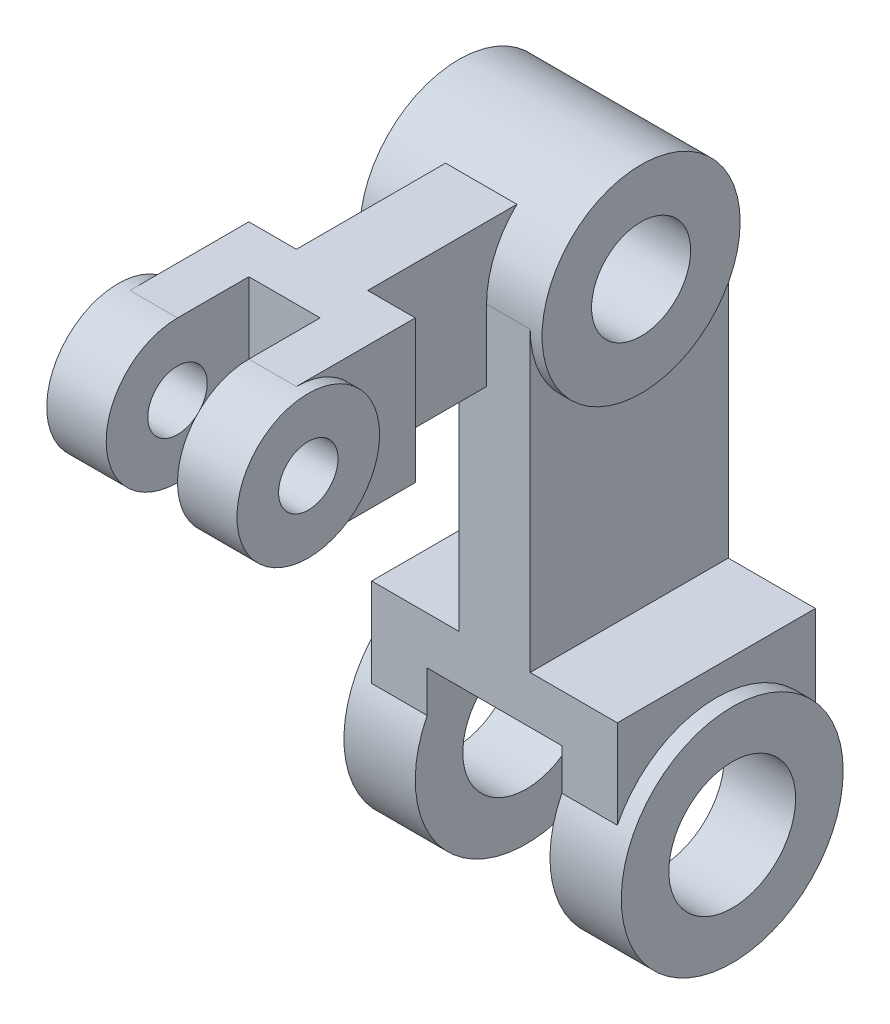
ISO-10303-21;
HEADER;
FILE_DESCRIPTION(('STEP AP214'),'2;1');
FILE_NAME('part.step','',(''),(''),'','','');
FILE_SCHEMA(('AUTOMOTIVE_DESIGN { 1 0 10303 214 1 1 1 1 }'));
ENDSEC;
DATA;
#1=APPLICATION_CONTEXT('core data for automotive mechanical design processes');
#2=APPLICATION_PROTOCOL_DEFINITION('international standard','automotive_design',2000,#1);
#3=PRODUCT_CONTEXT('',#1,'mechanical');
#4=PRODUCT('Part','Part','',(#3));
#5=PRODUCT_RELATED_PRODUCT_CATEGORY('part','',(#4));
#6=PRODUCT_DEFINITION_FORMATION('','',#4);
#7=PRODUCT_DEFINITION_CONTEXT('part definition',#1,'design');
#8=PRODUCT_DEFINITION('design','',#6,#7);
#9=PRODUCT_DEFINITION_SHAPE('','',#8);
#10=(LENGTH_UNIT() NAMED_UNIT(*) SI_UNIT(.MILLI.,.METRE.));
#11=(NAMED_UNIT(*) PLANE_ANGLE_UNIT() SI_UNIT($,.RADIAN.));
#12=(NAMED_UNIT(*) SI_UNIT($,.STERADIAN.) SOLID_ANGLE_UNIT());
#13=UNCERTAINTY_MEASURE_WITH_UNIT(LENGTH_MEASURE(1.E-05),#10,'distance_accuracy_value','');
#14=(GEOMETRIC_REPRESENTATION_CONTEXT(3) GLOBAL_UNCERTAINTY_ASSIGNED_CONTEXT((#13)) GLOBAL_UNIT_ASSIGNED_CONTEXT((#10,
#11,#12)) REPRESENTATION_CONTEXT('',''));
#15=CARTESIAN_POINT('',(0.,0.,0.));
#16=DIRECTION('',(0.,0.,1.));
#17=DIRECTION('',(1.,0.,0.));
#18=AXIS2_PLACEMENT_3D('',#15,#16,#17);
#19=CARTESIAN_POINT('',(13.,110.,85.));
#20=DIRECTION('',(-1.,0.,0.));
#21=DIRECTION('',(0.,0.,1.));
#22=AXIS2_PLACEMENT_3D('',#19,#20,#21);
#23=CYLINDRICAL_SURFACE('',#22,18.);
#24=CARTESIAN_POINT('',(-35.,110.,85.));
#25=DIRECTION('',(1.,0.,0.));
#26=DIRECTION('',(0.,0.,-1.));
#27=AXIS2_PLACEMENT_3D('',#24,#25,#26);
#28=CIRCLE('',#27,18.);
#29=CARTESIAN_POINT('',(-35.,110.,67.));
#30=VERTEX_POINT('',#29);
#31=EDGE_CURVE('E451',#30,#30,#28,.T.);
#32=ORIENTED_EDGE('',*,*,#31,.T.);
#33=EDGE_LOOP('',(#32));
#34=FACE_BOUND('',#33,.T.);
#35=CARTESIAN_POINT('',(-32.,110.,85.));
#36=DIRECTION('',(-1.,0.,0.));
#37=DIRECTION('',(0.,0.,1.));
#38=AXIS2_PLACEMENT_3D('',#35,#36,#37);
#39=CIRCLE('',#38,18.);
#40=CARTESIAN_POINT('',(-32.,128.,85.));
#41=VERTEX_POINT('',#40);
#42=CARTESIAN_POINT('',(-32.,92.,85.));
#43=VERTEX_POINT('',#42);
#44=EDGE_CURVE('E448',#41,#43,#39,.T.);
#45=ORIENTED_EDGE('',*,*,#44,.T.);
#46=DIRECTION('',(1.,0.,0.));
#47=VECTOR('',#46,1.);
#48=CARTESIAN_POINT('',(-20.,92.,85.));
#49=LINE('',#48,#47);
#50=CARTESIAN_POINT('',(-20.,92.,85.));
#51=VERTEX_POINT('',#50);
#52=EDGE_CURVE('E382',#43,#51,#49,.T.);
#53=ORIENTED_EDGE('',*,*,#52,.T.);
#54=CARTESIAN_POINT('',(-20.,110.,85.));
#55=DIRECTION('',(-1.,0.,0.));
#56=DIRECTION('',(0.,0.,1.));
#57=AXIS2_PLACEMENT_3D('',#54,#55,#56);
#58=CIRCLE('',#57,18.);
#59=CARTESIAN_POINT('',(-20.,128.,85.));
#60=VERTEX_POINT('',#59);
#61=EDGE_CURVE('E51',#51,#60,#58,.T.);
#62=ORIENTED_EDGE('',*,*,#61,.T.);
#63=DIRECTION('',(1.,0.,0.));
#64=VECTOR('',#63,1.);
#65=CARTESIAN_POINT('',(-20.,128.,85.));
#66=LINE('',#65,#64);
#67=EDGE_CURVE('E410',#41,#60,#66,.T.);
#68=ORIENTED_EDGE('',*,*,#67,.F.);
#69=EDGE_LOOP('',(#45,#53,#62,#68));
#70=FACE_BOUND('',#69,.T.);
#71=ADVANCED_FACE('F50',(#34,#70),#23,.T.);
#72=CARTESIAN_POINT('',(13.,110.,85.));
#73=DIRECTION('',(-1.,0.,0.));
#74=DIRECTION('',(0.,0.,1.));
#75=AXIS2_PLACEMENT_3D('',#72,#73,#74);
#76=CYLINDRICAL_SURFACE('',#75,7.5);
#77=CARTESIAN_POINT('',(-20.,110.,85.));
#78=DIRECTION('',(-1.,0.,0.));
#79=DIRECTION('',(0.,0.,1.));
#80=AXIS2_PLACEMENT_3D('',#77,#78,#79);
#81=CIRCLE('',#80,7.5);
#82=CARTESIAN_POINT('',(-20.,110.,92.5));
#83=VERTEX_POINT('',#82);
#84=EDGE_CURVE('E11',#83,#83,#81,.T.);
#85=ORIENTED_EDGE('',*,*,#84,.F.);
#86=EDGE_LOOP('',(#85));
#87=FACE_BOUND('',#86,.T.);
#88=CARTESIAN_POINT('',(-35.,110.,85.));
#89=DIRECTION('',(1.,0.,0.));
#90=DIRECTION('',(0.,0.,-1.));
#91=AXIS2_PLACEMENT_3D('',#88,#89,#90);
#92=CIRCLE('',#91,7.5);
#93=CARTESIAN_POINT('',(-35.,110.,77.5));
#94=VERTEX_POINT('',#93);
#95=EDGE_CURVE('E57',#94,#94,#92,.T.);
#96=ORIENTED_EDGE('',*,*,#95,.F.);
#97=EDGE_LOOP('',(#96));
#98=FACE_BOUND('',#97,.T.);
#99=ADVANCED_FACE('F47',(#87,#98),#76,.F.);
#100=CARTESIAN_POINT('',(-35.,110.,85.));
#101=DIRECTION('',(1.,0.,0.));
#102=DIRECTION('',(0.,0.,-1.));
#103=AXIS2_PLACEMENT_3D('',#100,#101,#102);
#104=PLANE('',#103);
#105=ORIENTED_EDGE('',*,*,#31,.F.);
#106=EDGE_LOOP('',(#105));
#107=FACE_BOUND('',#106,.T.);
#108=ORIENTED_EDGE('',*,*,#95,.T.);
#109=EDGE_LOOP('',(#108));
#110=FACE_BOUND('',#109,.T.);
#111=ADVANCED_FACE('F488',(#107,#110),#104,.F.);
#112=CARTESIAN_POINT('',(-20.,-28.,67.));
#113=DIRECTION('',(-1.,0.,0.));
#114=DIRECTION('',(0.,0.,1.));
#115=AXIS2_PLACEMENT_3D('',#112,#113,#114);
#116=PLANE('',#115);
#117=ORIENTED_EDGE('',*,*,#84,.T.);
#118=EDGE_LOOP('',(#117));
#119=FACE_BOUND('',#118,.T.);
#120=ORIENTED_EDGE('',*,*,#61,.F.);
#121=DIRECTION('',(0.,0.,-1.));
#122=VECTOR('',#121,1.);
#123=CARTESIAN_POINT('',(-20.,92.,85.));
#124=LINE('',#123,#122);
#125=CARTESIAN_POINT('',(-20.,92.,67.));
#126=VERTEX_POINT('',#125);
#127=EDGE_CURVE('E381',#51,#126,#124,.T.);
#128=ORIENTED_EDGE('',*,*,#127,.T.);
#129=DIRECTION('',(0.,1.,0.));
#130=VECTOR('',#129,1.);
#131=CARTESIAN_POINT('',(-20.,92.,67.));
#132=LINE('',#131,#130);
#133=CARTESIAN_POINT('',(-20.,128.,67.));
#134=VERTEX_POINT('',#133);
#135=EDGE_CURVE('E436',#126,#134,#132,.T.);
#136=ORIENTED_EDGE('',*,*,#135,.T.);
#137=DIRECTION('',(0.,0.,-1.));
#138=VECTOR('',#137,1.);
#139=CARTESIAN_POINT('',(-20.,128.,85.));
#140=LINE('',#139,#138);
#141=EDGE_CURVE('E407',#60,#134,#140,.T.);
#142=ORIENTED_EDGE('',*,*,#141,.F.);
#143=EDGE_LOOP('',(#120,#128,#136,#142));
#144=FACE_BOUND('',#143,.T.);
#145=ADVANCED_FACE('F465',(#119,#144),#116,.F.);
#146=CARTESIAN_POINT('',(-20.,92.,14.9257157700794));
#147=DIRECTION('',(-1.,0.,0.));
#148=DIRECTION('',(0.,0.,1.));
#149=AXIS2_PLACEMENT_3D('',#146,#147,#148);
#150=PLANE('',#149);
#151=CARTESIAN_POINT('',(-20.,110.,0.));
#152=DIRECTION('',(-1.,0.,0.));
#153=DIRECTION('',(0.,0.,1.));
#154=AXIS2_PLACEMENT_3D('',#151,#152,#153);
#155=CIRCLE('',#154,25.);
#156=CARTESIAN_POINT('',(-20.,92.,17.3493515728975));
#157=VERTEX_POINT('',#156);
#158=CARTESIAN_POINT('',(-20.,128.,17.3493515728975));
#159=VERTEX_POINT('',#158);
#160=EDGE_CURVE('E354',#157,#159,#155,.T.);
#161=ORIENTED_EDGE('',*,*,#160,.F.);
#162=DIRECTION('',(0.,0.,1.));
#163=VECTOR('',#162,1.);
#164=CARTESIAN_POINT('',(-20.,92.,14.9257157700794));
#165=LINE('',#164,#163);
#166=CARTESIAN_POINT('',(-20.,92.,55.));
#167=VERTEX_POINT('',#166);
#168=EDGE_CURVE('E375',#157,#167,#165,.T.);
#169=ORIENTED_EDGE('',*,*,#168,.T.);
#170=DIRECTION('',(0.,1.,0.));
#171=VECTOR('',#170,1.);
#172=CARTESIAN_POINT('',(-20.,92.,55.));
#173=LINE('',#172,#171);
#174=CARTESIAN_POINT('',(-20.,128.,55.));
#175=VERTEX_POINT('',#174);
#176=EDGE_CURVE('E401',#167,#175,#173,.T.);
#177=ORIENTED_EDGE('',*,*,#176,.T.);
#178=DIRECTION('',(0.,0.,1.));
#179=VECTOR('',#178,1.);
#180=CARTESIAN_POINT('',(-20.,128.,14.9257157700794));
#181=LINE('',#180,#179);
#182=EDGE_CURVE('E371',#159,#175,#181,.T.);
#183=ORIENTED_EDGE('',*,*,#182,.F.);
#184=EDGE_LOOP('',(#161,#169,#177,#183));
#185=FACE_BOUND('',#184,.T.);
#186=ADVANCED_FACE('F493',(#185),#150,.T.);
#187=CARTESIAN_POINT('',(-2.,92.,14.9257157700794));
#188=DIRECTION('',(1.,0.,0.));
#189=DIRECTION('',(0.,0.,-1.));
#190=AXIS2_PLACEMENT_3D('',#187,#188,#189);
#191=PLANE('',#190);
#192=CARTESIAN_POINT('',(-2.,110.,0.));
#193=DIRECTION('',(1.,0.,0.));
#194=DIRECTION('',(0.,0.,-1.));
#195=AXIS2_PLACEMENT_3D('',#192,#193,#194);
#196=CIRCLE('',#195,25.);
#197=CARTESIAN_POINT('',(-2.,128.,17.3493515728975));
#198=VERTEX_POINT('',#197);
#199=CARTESIAN_POINT('',(-2.,110.,25.));
#200=VERTEX_POINT('',#199);
#201=EDGE_CURVE('E348',#198,#200,#196,.T.);
#202=ORIENTED_EDGE('',*,*,#201,.F.);
#203=DIRECTION('',(0.,0.,-1.));
#204=VECTOR('',#203,1.);
#205=CARTESIAN_POINT('',(-2.,128.,14.9257157700794));
#206=LINE('',#205,#204);
#207=CARTESIAN_POINT('',(-2.,128.,55.));
#208=VERTEX_POINT('',#207);
#209=EDGE_CURVE('E374',#208,#198,#206,.T.);
#210=ORIENTED_EDGE('',*,*,#209,.F.);
#211=DIRECTION('',(0.,1.,0.));
#212=VECTOR('',#211,1.);
#213=CARTESIAN_POINT('',(-2.,92.,55.));
#214=LINE('',#213,#212);
#215=CARTESIAN_POINT('',(-2.,92.,55.));
#216=VERTEX_POINT('',#215);
#217=EDGE_CURVE('E429',#216,#208,#214,.T.);
#218=ORIENTED_EDGE('',*,*,#217,.F.);
#219=DIRECTION('',(0.,0.,-1.));
#220=VECTOR('',#219,1.);
#221=CARTESIAN_POINT('',(-2.,92.,14.9257157700794));
#222=LINE('',#221,#220);
#223=CARTESIAN_POINT('',(-2.,92.,25.));
#224=VERTEX_POINT('',#223);
#225=EDGE_CURVE('E402',#216,#224,#222,.T.);
#226=ORIENTED_EDGE('',*,*,#225,.T.);
#227=DIRECTION('',(0.,1.,0.));
#228=VECTOR('',#227,1.);
#229=CARTESIAN_POINT('',(-2.,92.,25.));
#230=LINE('',#229,#228);
#231=EDGE_CURVE('E71',#224,#200,#230,.T.);
#232=ORIENTED_EDGE('',*,*,#231,.T.);
#233=EDGE_LOOP('',(#202,#210,#218,#226,#232));
#234=FACE_BOUND('',#233,.T.);
#235=ADVANCED_FACE('F498',(#234),#191,.T.);
#236=CARTESIAN_POINT('',(10.,92.,55.));
#237=DIRECTION('',(0.,0.,-1.));
#238=DIRECTION('',(-1.,0.,0.));
#239=AXIS2_PLACEMENT_3D('',#236,#237,#238);
#240=PLANE('',#239);
#241=DIRECTION('',(-1.,0.,0.));
#242=VECTOR('',#241,1.);
#243=CARTESIAN_POINT('',(10.,128.,55.));
#244=LINE('',#243,#242);
#245=CARTESIAN_POINT('',(10.,128.,55.));
#246=VERTEX_POINT('',#245);
#247=EDGE_CURVE('E424',#246,#208,#244,.T.);
#248=ORIENTED_EDGE('',*,*,#247,.F.);
#249=DIRECTION('',(0.,1.,0.));
#250=VECTOR('',#249,1.);
#251=CARTESIAN_POINT('',(10.,92.,55.));
#252=LINE('',#251,#250);
#253=CARTESIAN_POINT('',(10.,92.,55.));
#254=VERTEX_POINT('',#253);
#255=EDGE_CURVE('E435',#254,#246,#252,.T.);
#256=ORIENTED_EDGE('',*,*,#255,.F.);
#257=DIRECTION('',(-1.,0.,0.));
#258=VECTOR('',#257,1.);
#259=CARTESIAN_POINT('',(10.,92.,55.));
#260=LINE('',#259,#258);
#261=EDGE_CURVE('E400',#254,#216,#260,.T.);
#262=ORIENTED_EDGE('',*,*,#261,.T.);
#263=ORIENTED_EDGE('',*,*,#217,.T.);
#264=EDGE_LOOP('',(#248,#256,#262,#263));
#265=FACE_BOUND('',#264,.T.);
#266=ADVANCED_FACE('F520',(#265),#240,.T.);
#267=CARTESIAN_POINT('',(10.,92.,85.));
#268=DIRECTION('',(1.,0.,0.));
#269=DIRECTION('',(0.,0.,-1.));
#270=AXIS2_PLACEMENT_3D('',#267,#268,#269);
#271=PLANE('',#270);
#272=DIRECTION('',(0.,0.,-1.));
#273=VECTOR('',#272,1.);
#274=CARTESIAN_POINT('',(10.,128.,85.));
#275=LINE('',#274,#273);
#276=CARTESIAN_POINT('',(10.,128.,85.));
#277=VERTEX_POINT('',#276);
#278=EDGE_CURVE('E422',#277,#246,#275,.T.);
#279=ORIENTED_EDGE('',*,*,#278,.F.);
#280=CARTESIAN_POINT('',(10.,110.,85.));
#281=DIRECTION('',(1.,0.,0.));
#282=DIRECTION('',(0.,0.,-1.));
#283=AXIS2_PLACEMENT_3D('',#280,#281,#282);
#284=CIRCLE('',#283,18.);
#285=CARTESIAN_POINT('',(10.,92.,85.));
#286=VERTEX_POINT('',#285);
#287=EDGE_CURVE('E366',#277,#286,#284,.F.);
#288=ORIENTED_EDGE('',*,*,#287,.T.);
#289=DIRECTION('',(0.,0.,-1.));
#290=VECTOR('',#289,1.);
#291=CARTESIAN_POINT('',(10.,92.,85.));
#292=LINE('',#291,#290);
#293=EDGE_CURVE('E395',#286,#254,#292,.T.);
#294=ORIENTED_EDGE('',*,*,#293,.T.);
#295=ORIENTED_EDGE('',*,*,#255,.T.);
#296=EDGE_LOOP('',(#279,#288,#294,#295));
#297=FACE_BOUND('',#296,.T.);
#298=ADVANCED_FACE('F511',(#297),#271,.T.);
#299=CARTESIAN_POINT('',(-1.99999999999999,92.,85.));
#300=DIRECTION('',(-1.,0.,0.));
#301=DIRECTION('',(0.,0.,1.));
#302=AXIS2_PLACEMENT_3D('',#299,#300,#301);
#303=PLANE('',#302);
#304=CARTESIAN_POINT('',(-1.99999999999999,110.,85.));
#305=DIRECTION('',(1.,0.,0.));
#306=DIRECTION('',(0.,0.,-1.));
#307=AXIS2_PLACEMENT_3D('',#304,#305,#306);
#308=CIRCLE('',#307,7.5);
#309=CARTESIAN_POINT('',(-1.99999999999999,110.,77.5));
#310=VERTEX_POINT('',#309);
#311=EDGE_CURVE('E357',#310,#310,#308,.T.);
#312=ORIENTED_EDGE('',*,*,#311,.T.);
#313=EDGE_LOOP('',(#312));
#314=FACE_BOUND('',#313,.T.);
#315=DIRECTION('',(0.,0.,1.));
#316=VECTOR('',#315,1.);
#317=CARTESIAN_POINT('',(-1.99999999999999,92.,85.));
#318=LINE('',#317,#316);
#319=CARTESIAN_POINT('',(-1.99999999999999,92.,67.));
#320=VERTEX_POINT('',#319);
#321=CARTESIAN_POINT('',(-1.99999999999999,92.,85.));
#322=VERTEX_POINT('',#321);
#323=EDGE_CURVE('E387',#320,#322,#318,.T.);
#324=ORIENTED_EDGE('',*,*,#323,.T.);
#325=CARTESIAN_POINT('',(-1.99999999999999,110.,85.));
#326=DIRECTION('',(1.,0.,0.));
#327=DIRECTION('',(0.,0.,-1.));
#328=AXIS2_PLACEMENT_3D('',#325,#326,#327);
#329=CIRCLE('',#328,18.);
#330=CARTESIAN_POINT('',(-1.99999999999999,128.,85.));
#331=VERTEX_POINT('',#330);
#332=EDGE_CURVE('E356',#331,#322,#329,.T.);
#333=ORIENTED_EDGE('',*,*,#332,.F.);
#334=DIRECTION('',(0.,0.,1.));
#335=VECTOR('',#334,1.);
#336=CARTESIAN_POINT('',(-1.99999999999999,128.,85.));
#337=LINE('',#336,#335);
#338=CARTESIAN_POINT('',(-1.99999999999999,128.,67.));
#339=VERTEX_POINT('',#338);
#340=EDGE_CURVE('E419',#339,#331,#337,.T.);
#341=ORIENTED_EDGE('',*,*,#340,.F.);
#342=DIRECTION('',(0.,1.,0.));
#343=VECTOR('',#342,1.);
#344=CARTESIAN_POINT('',(-1.99999999999999,92.,67.));
#345=LINE('',#344,#343);
#346=EDGE_CURVE('E432',#320,#339,#345,.T.);
#347=ORIENTED_EDGE('',*,*,#346,.F.);
#348=EDGE_LOOP('',(#324,#333,#341,#347));
#349=FACE_BOUND('',#348,.T.);
#350=ADVANCED_FACE('F509',(#314,#349),#303,.T.);
#351=CARTESIAN_POINT('',(-20.,92.,67.));
#352=DIRECTION('',(0.,0.,1.));
#353=DIRECTION('',(1.,0.,0.));
#354=AXIS2_PLACEMENT_3D('',#351,#352,#353);
#355=PLANE('',#354);
#356=DIRECTION('',(1.,0.,0.));
#357=VECTOR('',#356,1.);
#358=CARTESIAN_POINT('',(-20.,128.,67.));
#359=LINE('',#358,#357);
#360=EDGE_CURVE('E414',#134,#339,#359,.T.);
#361=ORIENTED_EDGE('',*,*,#360,.F.);
#362=ORIENTED_EDGE('',*,*,#135,.F.);
#363=DIRECTION('',(1.,0.,0.));
#364=VECTOR('',#363,1.);
#365=CARTESIAN_POINT('',(-20.,92.,67.));
#366=LINE('',#365,#364);
#367=EDGE_CURVE('E386',#126,#320,#366,.T.);
#368=ORIENTED_EDGE('',*,*,#367,.T.);
#369=ORIENTED_EDGE('',*,*,#346,.T.);
#370=EDGE_LOOP('',(#361,#362,#368,#369));
#371=FACE_BOUND('',#370,.T.);
#372=ADVANCED_FACE('F506',(#371),#355,.T.);
#373=CARTESIAN_POINT('',(-32.,92.,85.));
#374=DIRECTION('',(-1.,0.,0.));
#375=DIRECTION('',(0.,0.,1.));
#376=AXIS2_PLACEMENT_3D('',#373,#374,#375);
#377=PLANE('',#376);
#378=ORIENTED_EDGE('',*,*,#44,.F.);
#379=DIRECTION('',(0.,0.,1.));
#380=VECTOR('',#379,1.);
#381=CARTESIAN_POINT('',(-32.,128.,85.));
#382=LINE('',#381,#380);
#383=CARTESIAN_POINT('',(-32.,128.,55.));
#384=VERTEX_POINT('',#383);
#385=EDGE_CURVE('E63',#384,#41,#382,.T.);
#386=ORIENTED_EDGE('',*,*,#385,.F.);
#387=DIRECTION('',(0.,1.,0.));
#388=VECTOR('',#387,1.);
#389=CARTESIAN_POINT('',(-32.,92.,55.));
#390=LINE('',#389,#388);
#391=CARTESIAN_POINT('',(-32.,92.,55.));
#392=VERTEX_POINT('',#391);
#393=EDGE_CURVE('E438',#392,#384,#390,.T.);
#394=ORIENTED_EDGE('',*,*,#393,.F.);
#395=DIRECTION('',(0.,0.,1.));
#396=VECTOR('',#395,1.);
#397=CARTESIAN_POINT('',(-32.,92.,85.));
#398=LINE('',#397,#396);
#399=EDGE_CURVE('E377',#392,#43,#398,.T.);
#400=ORIENTED_EDGE('',*,*,#399,.T.);
#401=EDGE_LOOP('',(#378,#386,#394,#400));
#402=FACE_BOUND('',#401,.T.);
#403=ADVANCED_FACE('F505',(#402),#377,.T.);
#404=CARTESIAN_POINT('',(-32.,92.,55.));
#405=DIRECTION('',(0.,0.,-1.));
#406=DIRECTION('',(-1.,0.,0.));
#407=AXIS2_PLACEMENT_3D('',#404,#405,#406);
#408=PLANE('',#407);
#409=DIRECTION('',(-1.,0.,0.));
#410=VECTOR('',#409,1.);
#411=CARTESIAN_POINT('',(-32.,128.,55.));
#412=LINE('',#411,#410);
#413=EDGE_CURVE('E403',#175,#384,#412,.T.);
#414=ORIENTED_EDGE('',*,*,#413,.F.);
#415=ORIENTED_EDGE('',*,*,#176,.F.);
#416=DIRECTION('',(-1.,0.,0.));
#417=VECTOR('',#416,1.);
#418=CARTESIAN_POINT('',(-32.,92.,55.));
#419=LINE('',#418,#417);
#420=EDGE_CURVE('E372',#167,#392,#419,.T.);
#421=ORIENTED_EDGE('',*,*,#420,.T.);
#422=ORIENTED_EDGE('',*,*,#393,.T.);
#423=EDGE_LOOP('',(#414,#415,#421,#422));
#424=FACE_BOUND('',#423,.T.);
#425=ADVANCED_FACE('F477',(#424),#408,.T.);
#426=CARTESIAN_POINT('',(0.,92.,0.));
#427=DIRECTION('',(0.,1.,0.));
#428=DIRECTION('',(0.,0.,1.));
#429=AXIS2_PLACEMENT_3D('',#426,#427,#428);
#430=PLANE('',#429);
#431=ORIENTED_EDGE('',*,*,#168,.F.);
#432=DIRECTION('',(1.,0.,0.));
#433=VECTOR('',#432,1.);
#434=CARTESIAN_POINT('',(-34.,92.,17.3493515728975));
#435=LINE('',#434,#433);
#436=CARTESIAN_POINT('',(-9.,92.,17.3493515728975));
#437=VERTEX_POINT('',#436);
#438=EDGE_CURVE('E353',#157,#437,#435,.T.);
#439=ORIENTED_EDGE('',*,*,#438,.T.);
#440=DIRECTION('',(0.,0.,-1.));
#441=VECTOR('',#440,1.);
#442=CARTESIAN_POINT('',(-9.,92.,0.));
#443=LINE('',#442,#441);
#444=CARTESIAN_POINT('',(-9.,92.,25.));
#445=VERTEX_POINT('',#444);
#446=EDGE_CURVE('E450',#445,#437,#443,.T.);
#447=ORIENTED_EDGE('',*,*,#446,.F.);
#448=DIRECTION('',(-1.,0.,0.));
#449=VECTOR('',#448,1.);
#450=CARTESIAN_POINT('',(0.,92.,25.));
#451=LINE('',#450,#449);
#452=EDGE_CURVE('E443',#224,#445,#451,.T.);
#453=ORIENTED_EDGE('',*,*,#452,.F.);
#454=ORIENTED_EDGE('',*,*,#225,.F.);
#455=ORIENTED_EDGE('',*,*,#261,.F.);
#456=ORIENTED_EDGE('',*,*,#293,.F.);
#457=DIRECTION('',(1.,0.,0.));
#458=VECTOR('',#457,1.);
#459=CARTESIAN_POINT('',(-1.99999999999999,92.,85.));
#460=LINE('',#459,#458);
#461=EDGE_CURVE('E394',#322,#286,#460,.T.);
#462=ORIENTED_EDGE('',*,*,#461,.F.);
#463=ORIENTED_EDGE('',*,*,#323,.F.);
#464=ORIENTED_EDGE('',*,*,#367,.F.);
#465=ORIENTED_EDGE('',*,*,#127,.F.);
#466=ORIENTED_EDGE('',*,*,#52,.F.);
#467=ORIENTED_EDGE('',*,*,#399,.F.);
#468=ORIENTED_EDGE('',*,*,#420,.F.);
#469=EDGE_LOOP('',(#431,#439,#447,#453,#454,#455,#456,#462,#463,#464,#465,#466,#467,#468));
#470=FACE_BOUND('',#469,.T.);
#471=ADVANCED_FACE('F469',(#470),#430,.F.);
#472=CARTESIAN_POINT('',(0.,128.,0.));
#473=DIRECTION('',(0.,1.,0.));
#474=DIRECTION('',(0.,0.,1.));
#475=AXIS2_PLACEMENT_3D('',#472,#473,#474);
#476=PLANE('',#475);
#477=DIRECTION('',(1.,0.,0.));
#478=VECTOR('',#477,1.);
#479=CARTESIAN_POINT('',(-34.,128.,17.3493515728975));
#480=LINE('',#479,#478);
#481=EDGE_CURVE('E431',#159,#198,#480,.T.);
#482=ORIENTED_EDGE('',*,*,#481,.F.);
#483=ORIENTED_EDGE('',*,*,#182,.T.);
#484=ORIENTED_EDGE('',*,*,#413,.T.);
#485=ORIENTED_EDGE('',*,*,#385,.T.);
#486=ORIENTED_EDGE('',*,*,#67,.T.);
#487=ORIENTED_EDGE('',*,*,#141,.T.);
#488=ORIENTED_EDGE('',*,*,#360,.T.);
#489=ORIENTED_EDGE('',*,*,#340,.T.);
#490=DIRECTION('',(1.,0.,0.));
#491=VECTOR('',#490,1.);
#492=CARTESIAN_POINT('',(-1.99999999999999,128.,85.));
#493=LINE('',#492,#491);
#494=EDGE_CURVE('E418',#331,#277,#493,.T.);
#495=ORIENTED_EDGE('',*,*,#494,.T.);
#496=ORIENTED_EDGE('',*,*,#278,.T.);
#497=ORIENTED_EDGE('',*,*,#247,.T.);
#498=ORIENTED_EDGE('',*,*,#209,.T.);
#499=EDGE_LOOP('',(#482,#483,#484,#485,#486,#487,#488,#489,#495,#496,#497,#498));
#500=FACE_BOUND('',#499,.T.);
#501=ADVANCED_FACE('F462',(#500),#476,.T.);
#502=CARTESIAN_POINT('',(13.,110.,85.));
#503=DIRECTION('',(-1.,0.,0.));
#504=DIRECTION('',(0.,0.,1.));
#505=AXIS2_PLACEMENT_3D('',#502,#503,#504);
#506=CYLINDRICAL_SURFACE('',#505,18.);
#507=CARTESIAN_POINT('',(13.,110.,85.));
#508=DIRECTION('',(1.,0.,0.));
#509=DIRECTION('',(0.,0.,-1.));
#510=AXIS2_PLACEMENT_3D('',#507,#508,#509);
#511=CIRCLE('',#510,18.);
#512=CARTESIAN_POINT('',(13.,110.,67.));
#513=VERTEX_POINT('',#512);
#514=EDGE_CURVE('E361',#513,#513,#511,.T.);
#515=ORIENTED_EDGE('',*,*,#514,.F.);
#516=EDGE_LOOP('',(#515));
#517=FACE_BOUND('',#516,.T.);
#518=ORIENTED_EDGE('',*,*,#332,.T.);
#519=ORIENTED_EDGE('',*,*,#461,.T.);
#520=ORIENTED_EDGE('',*,*,#287,.F.);
#521=ORIENTED_EDGE('',*,*,#494,.F.);
#522=EDGE_LOOP('',(#518,#519,#520,#521));
#523=FACE_BOUND('',#522,.T.);
#524=ADVANCED_FACE('F466',(#517,#523),#506,.T.);
#525=CARTESIAN_POINT('',(13.,110.,85.));
#526=DIRECTION('',(1.,0.,0.));
#527=DIRECTION('',(0.,0.,-1.));
#528=AXIS2_PLACEMENT_3D('',#525,#526,#527);
#529=PLANE('',#528);
#530=ORIENTED_EDGE('',*,*,#514,.T.);
#531=EDGE_LOOP('',(#530));
#532=FACE_BOUND('',#531,.T.);
#533=CARTESIAN_POINT('',(13.,110.,85.));
#534=DIRECTION('',(1.,0.,0.));
#535=DIRECTION('',(0.,0.,-1.));
#536=AXIS2_PLACEMENT_3D('',#533,#534,#535);
#537=CIRCLE('',#536,7.5);
#538=CARTESIAN_POINT('',(13.,110.,77.5));
#539=VERTEX_POINT('',#538);
#540=EDGE_CURVE('E359',#539,#539,#537,.T.);
#541=ORIENTED_EDGE('',*,*,#540,.F.);
#542=EDGE_LOOP('',(#541));
#543=FACE_BOUND('',#542,.T.);
#544=ADVANCED_FACE('F473',(#532,#543),#529,.T.);
#545=CARTESIAN_POINT('',(13.,110.,85.));
#546=DIRECTION('',(-1.,0.,0.));
#547=DIRECTION('',(0.,0.,1.));
#548=AXIS2_PLACEMENT_3D('',#545,#546,#547);
#549=CYLINDRICAL_SURFACE('',#548,7.5);
#550=ORIENTED_EDGE('',*,*,#311,.F.);
#551=EDGE_LOOP('',(#550));
#552=FACE_BOUND('',#551,.T.);
#553=ORIENTED_EDGE('',*,*,#540,.T.);
#554=EDGE_LOOP('',(#553));
#555=FACE_BOUND('',#554,.T.);
#556=ADVANCED_FACE('F599',(#552,#555),#549,.F.);
#557=CARTESIAN_POINT('',(-9.,135.002,25.));
#558=DIRECTION('',(1.,0.,0.));
#559=DIRECTION('',(0.,0.,-1.));
#560=AXIS2_PLACEMENT_3D('',#557,#558,#559);
#561=PLANE('',#560);
#562=DIRECTION('',(0.,-1.,0.));
#563=VECTOR('',#562,1.);
#564=CARTESIAN_POINT('',(-9.,135.002,25.));
#565=LINE('',#564,#563);
#566=CARTESIAN_POINT('',(-9.,35.,25.));
#567=VERTEX_POINT('',#566);
#568=EDGE_CURVE('E322',#445,#567,#565,.T.);
#569=ORIENTED_EDGE('',*,*,#568,.F.);
#570=ORIENTED_EDGE('',*,*,#446,.T.);
#571=CARTESIAN_POINT('',(-9.,110.,0.));
#572=DIRECTION('',(1.,0.,0.));
#573=DIRECTION('',(0.,0.,-1.));
#574=AXIS2_PLACEMENT_3D('',#571,#572,#573);
#575=CIRCLE('',#574,25.);
#576=CARTESIAN_POINT('',(-9.,110.,-25.));
#577=VERTEX_POINT('',#576);
#578=EDGE_CURVE('E320',#437,#577,#575,.T.);
#579=ORIENTED_EDGE('',*,*,#578,.T.);
#580=DIRECTION('',(0.,-1.,0.));
#581=VECTOR('',#580,1.);
#582=CARTESIAN_POINT('',(-9.,135.002,-25.));
#583=LINE('',#582,#581);
#584=CARTESIAN_POINT('',(-9.,35.,-25.));
#585=VERTEX_POINT('',#584);
#586=EDGE_CURVE('E321',#577,#585,#583,.T.);
#587=ORIENTED_EDGE('',*,*,#586,.T.);
#588=DIRECTION('',(0.,0.,1.));
#589=VECTOR('',#588,1.);
#590=CARTESIAN_POINT('',(-9.,35.,25.));
#591=LINE('',#590,#589);
#592=EDGE_CURVE('E306',#585,#567,#591,.T.);
#593=ORIENTED_EDGE('',*,*,#592,.T.);
#594=EDGE_LOOP('',(#569,#570,#579,#587,#593));
#595=FACE_BOUND('',#594,.T.);
#596=ADVANCED_FACE('F552',(#595),#561,.F.);
#597=CARTESIAN_POINT('',(-34.,110.,0.));
#598=DIRECTION('',(1.,0.,0.));
#599=DIRECTION('',(0.,0.,-1.));
#600=AXIS2_PLACEMENT_3D('',#597,#598,#599);
#601=CYLINDRICAL_SURFACE('',#600,25.);
#602=CARTESIAN_POINT('',(12.,110.,0.));
#603=DIRECTION('',(1.,0.,0.));
#604=DIRECTION('',(0.,0.,-1.));
#605=AXIS2_PLACEMENT_3D('',#602,#603,#604);
#606=CIRCLE('',#605,25.);
#607=CARTESIAN_POINT('',(12.,110.,-25.));
#608=VERTEX_POINT('',#607);
#609=EDGE_CURVE('E337',#608,#608,#606,.T.);
#610=ORIENTED_EDGE('',*,*,#609,.F.);
#611=EDGE_LOOP('',(#610));
#612=FACE_BOUND('',#611,.T.);
#613=CARTESIAN_POINT('',(-34.,110.,0.));
#614=DIRECTION('',(1.,0.,0.));
#615=DIRECTION('',(0.,0.,-1.));
#616=AXIS2_PLACEMENT_3D('',#613,#614,#615);
#617=CIRCLE('',#616,25.);
#618=CARTESIAN_POINT('',(-34.,110.,-25.));
#619=VERTEX_POINT('',#618);
#620=EDGE_CURVE('E339',#619,#619,#617,.T.);
#621=ORIENTED_EDGE('',*,*,#620,.T.);
#622=EDGE_LOOP('',(#621));
#623=FACE_BOUND('',#622,.T.);
#624=ORIENTED_EDGE('',*,*,#438,.F.);
#625=ORIENTED_EDGE('',*,*,#160,.T.);
#626=ORIENTED_EDGE('',*,*,#481,.T.);
#627=ORIENTED_EDGE('',*,*,#201,.T.);
#628=DIRECTION('',(1.,0.,0.));
#629=VECTOR('',#628,1.);
#630=CARTESIAN_POINT('',(-34.,110.,25.));
#631=LINE('',#630,#629);
#632=CARTESIAN_POINT('',(9.,110.,25.));
#633=VERTEX_POINT('',#632);
#634=EDGE_CURVE('E303',#200,#633,#631,.T.);
#635=ORIENTED_EDGE('',*,*,#634,.T.);
#636=CARTESIAN_POINT('',(9.,110.,0.));
#637=DIRECTION('',(-1.,0.,0.));
#638=DIRECTION('',(0.,0.,1.));
#639=AXIS2_PLACEMENT_3D('',#636,#637,#638);
#640=CIRCLE('',#639,25.);
#641=CARTESIAN_POINT('',(9.,110.,-25.));
#642=VERTEX_POINT('',#641);
#643=EDGE_CURVE('E319',#642,#633,#640,.T.);
#644=ORIENTED_EDGE('',*,*,#643,.F.);
#645=DIRECTION('',(1.,0.,0.));
#646=VECTOR('',#645,1.);
#647=CARTESIAN_POINT('',(-34.,110.,-25.));
#648=LINE('',#647,#646);
#649=EDGE_CURVE('E313',#577,#642,#648,.T.);
#650=ORIENTED_EDGE('',*,*,#649,.F.);
#651=ORIENTED_EDGE('',*,*,#578,.F.);
#652=EDGE_LOOP('',(#624,#625,#626,#627,#635,#644,#650,#651));
#653=FACE_BOUND('',#652,.T.);
#654=ADVANCED_FACE('F530',(#612,#623,#653),#601,.T.);
#655=CARTESIAN_POINT('',(35.,0.,0.));
#656=DIRECTION('',(-1.,0.,0.));
#657=DIRECTION('',(0.,0.,1.));
#658=AXIS2_PLACEMENT_3D('',#655,#656,#657);
#659=CYLINDRICAL_SURFACE('',#658,28.);
#660=CARTESIAN_POINT('',(35.,0.,0.));
#661=DIRECTION('',(1.,0.,0.));
#662=DIRECTION('',(0.,0.,-1.));
#663=AXIS2_PLACEMENT_3D('',#660,#661,#662);
#664=CIRCLE('',#663,28.);
#665=CARTESIAN_POINT('',(35.,0.,-28.));
#666=VERTEX_POINT('',#665);
#667=EDGE_CURVE('E297',#666,#666,#664,.T.);
#668=ORIENTED_EDGE('',*,*,#667,.F.);
#669=EDGE_LOOP('',(#668));
#670=FACE_BOUND('',#669,.T.);
#671=DIRECTION('',(-1.,0.,0.));
#672=VECTOR('',#671,1.);
#673=CARTESIAN_POINT('',(35.,12.6095202129185,25.));
#674=LINE('',#673,#672);
#675=CARTESIAN_POINT('',(17.,12.6095202129185,25.));
#676=VERTEX_POINT('',#675);
#677=CARTESIAN_POINT('',(31.,12.6095202129185,25.));
#678=VERTEX_POINT('',#677);
#679=EDGE_CURVE('E266',#676,#678,#674,.F.);
#680=ORIENTED_EDGE('',*,*,#679,.F.);
#681=CARTESIAN_POINT('',(17.,0.,0.));
#682=DIRECTION('',(1.,0.,0.));
#683=DIRECTION('',(0.,1.,0.));
#684=AXIS2_PLACEMENT_3D('',#681,#682,#683);
#685=CIRCLE('',#684,28.);
#686=CARTESIAN_POINT('',(17.,12.6095202129185,-25.));
#687=VERTEX_POINT('',#686);
#688=EDGE_CURVE('E252',#676,#687,#685,.T.);
#689=ORIENTED_EDGE('',*,*,#688,.T.);
#690=DIRECTION('',(-1.,0.,0.));
#691=VECTOR('',#690,1.);
#692=CARTESIAN_POINT('',(35.,12.6095202129185,-25.));
#693=LINE('',#692,#691);
#694=CARTESIAN_POINT('',(31.,12.6095202129185,-25.));
#695=VERTEX_POINT('',#694);
#696=EDGE_CURVE('E244',#695,#687,#693,.T.);
#697=ORIENTED_EDGE('',*,*,#696,.F.);
#698=CARTESIAN_POINT('',(31.,0.,0.));
#699=DIRECTION('',(1.,0.,0.));
#700=DIRECTION('',(0.,0.,-1.));
#701=AXIS2_PLACEMENT_3D('',#698,#699,#700);
#702=CIRCLE('',#701,28.);
#703=EDGE_CURVE('E233',#678,#695,#702,.F.);
#704=ORIENTED_EDGE('',*,*,#703,.F.);
#705=EDGE_LOOP('',(#680,#689,#697,#704));
#706=FACE_BOUND('',#705,.T.);
#707=ADVANCED_FACE('F572',(#670,#706),#659,.T.);
#708=CARTESIAN_POINT('',(35.,0.,0.));
#709=DIRECTION('',(-1.,0.,0.));
#710=DIRECTION('',(0.,0.,1.));
#711=AXIS2_PLACEMENT_3D('',#708,#709,#710);
#712=CYLINDRICAL_SURFACE('',#711,16.);
#713=CARTESIAN_POINT('',(-17.,0.,0.));
#714=DIRECTION('',(-1.,0.,0.));
#715=DIRECTION('',(0.,-1.,0.));
#716=AXIS2_PLACEMENT_3D('',#713,#714,#715);
#717=CIRCLE('',#716,16.);
#718=CARTESIAN_POINT('',(-17.,-16.,0.));
#719=VERTEX_POINT('',#718);
#720=EDGE_CURVE('E246',#719,#719,#717,.T.);
#721=ORIENTED_EDGE('',*,*,#720,.F.);
#722=EDGE_LOOP('',(#721));
#723=FACE_BOUND('',#722,.T.);
#724=CARTESIAN_POINT('',(-35.,0.,0.));
#725=DIRECTION('',(1.,0.,0.));
#726=DIRECTION('',(0.,0.,-1.));
#727=AXIS2_PLACEMENT_3D('',#724,#725,#726);
#728=CIRCLE('',#727,16.);
#729=CARTESIAN_POINT('',(-35.,0.,-16.));
#730=VERTEX_POINT('',#729);
#731=EDGE_CURVE('E280',#730,#730,#728,.T.);
#732=ORIENTED_EDGE('',*,*,#731,.F.);
#733=EDGE_LOOP('',(#732));
#734=FACE_BOUND('',#733,.T.);
#735=ADVANCED_FACE('F609',(#723,#734),#712,.F.);
#736=CARTESIAN_POINT('',(-34.,110.,0.));
#737=DIRECTION('',(1.,0.,0.));
#738=DIRECTION('',(0.,0.,-1.));
#739=AXIS2_PLACEMENT_3D('',#736,#737,#738);
#740=PLANE('',#739);
#741=CARTESIAN_POINT('',(-34.,110.,0.));
#742=DIRECTION('',(1.,0.,0.));
#743=DIRECTION('',(0.,0.,-1.));
#744=AXIS2_PLACEMENT_3D('',#741,#742,#743);
#745=CIRCLE('',#744,12.5);
#746=CARTESIAN_POINT('',(-34.,110.,-12.5));
#747=VERTEX_POINT('',#746);
#748=EDGE_CURVE('E335',#747,#747,#745,.T.);
#749=ORIENTED_EDGE('',*,*,#748,.T.);
#750=EDGE_LOOP('',(#749));
#751=FACE_BOUND('',#750,.T.);
#752=ORIENTED_EDGE('',*,*,#620,.F.);
#753=EDGE_LOOP('',(#752));
#754=FACE_BOUND('',#753,.T.);
#755=ADVANCED_FACE('F602',(#751,#754),#740,.F.);
#756=CARTESIAN_POINT('',(12.,110.,0.));
#757=DIRECTION('',(1.,0.,0.));
#758=DIRECTION('',(0.,0.,-1.));
#759=AXIS2_PLACEMENT_3D('',#756,#757,#758);
#760=PLANE('',#759);
#761=CARTESIAN_POINT('',(12.,110.,0.));
#762=DIRECTION('',(1.,0.,0.));
#763=DIRECTION('',(0.,0.,-1.));
#764=AXIS2_PLACEMENT_3D('',#761,#762,#763);
#765=CIRCLE('',#764,12.5);
#766=CARTESIAN_POINT('',(12.,110.,-12.5));
#767=VERTEX_POINT('',#766);
#768=EDGE_CURVE('E312',#767,#767,#765,.T.);
#769=ORIENTED_EDGE('',*,*,#768,.F.);
#770=EDGE_LOOP('',(#769));
#771=FACE_BOUND('',#770,.T.);
#772=ORIENTED_EDGE('',*,*,#609,.T.);
#773=EDGE_LOOP('',(#772));
#774=FACE_BOUND('',#773,.T.);
#775=ADVANCED_FACE('F605',(#771,#774),#760,.T.);
#776=CARTESIAN_POINT('',(-34.,110.,0.));
#777=DIRECTION('',(1.,0.,0.));
#778=DIRECTION('',(0.,0.,-1.));
#779=AXIS2_PLACEMENT_3D('',#776,#777,#778);
#780=CYLINDRICAL_SURFACE('',#779,12.5);
#781=ORIENTED_EDGE('',*,*,#748,.F.);
#782=EDGE_LOOP('',(#781));
#783=FACE_BOUND('',#782,.T.);
#784=ORIENTED_EDGE('',*,*,#768,.T.);
#785=EDGE_LOOP('',(#784));
#786=FACE_BOUND('',#785,.T.);
#787=ADVANCED_FACE('F593',(#783,#786),#780,.F.);
#788=CARTESIAN_POINT('',(-9.,135.002,-25.));
#789=DIRECTION('',(0.,0.,1.));
#790=DIRECTION('',(1.,0.,0.));
#791=AXIS2_PLACEMENT_3D('',#788,#789,#790);
#792=PLANE('',#791);
#793=DIRECTION('',(-1.,0.,0.));
#794=VECTOR('',#793,1.);
#795=CARTESIAN_POINT('',(-9.,23.,-25.));
#796=LINE('',#795,#794);
#797=CARTESIAN_POINT('',(17.,23.,-25.));
#798=VERTEX_POINT('',#797);
#799=CARTESIAN_POINT('',(-17.,23.,-25.));
#800=VERTEX_POINT('',#799);
#801=EDGE_CURVE('E224',#798,#800,#796,.T.);
#802=ORIENTED_EDGE('',*,*,#801,.T.);
#803=DIRECTION('',(0.,-1.,0.));
#804=VECTOR('',#803,1.);
#805=CARTESIAN_POINT('',(-17.,135.002,-25.));
#806=LINE('',#805,#804);
#807=CARTESIAN_POINT('',(-17.,12.6095202129185,-25.));
#808=VERTEX_POINT('',#807);
#809=EDGE_CURVE('E235',#800,#808,#806,.T.);
#810=ORIENTED_EDGE('',*,*,#809,.T.);
#811=CARTESIAN_POINT('',(-31.,12.6095202129185,-25.));
#812=VERTEX_POINT('',#811);
#813=EDGE_CURVE('E262',#808,#812,#693,.T.);
#814=ORIENTED_EDGE('',*,*,#813,.T.);
#815=DIRECTION('',(0.,1.,0.));
#816=VECTOR('',#815,1.);
#817=CARTESIAN_POINT('',(-31.,-28.002,-25.));
#818=LINE('',#817,#816);
#819=CARTESIAN_POINT('',(-31.,35.,-25.));
#820=VERTEX_POINT('',#819);
#821=EDGE_CURVE('E284',#812,#820,#818,.T.);
#822=ORIENTED_EDGE('',*,*,#821,.T.);
#823=DIRECTION('',(-1.,0.,0.));
#824=VECTOR('',#823,1.);
#825=CARTESIAN_POINT('',(-31.,35.,-25.));
#826=LINE('',#825,#824);
#827=EDGE_CURVE('E272',#585,#820,#826,.T.);
#828=ORIENTED_EDGE('',*,*,#827,.F.);
#829=ORIENTED_EDGE('',*,*,#586,.F.);
#830=ORIENTED_EDGE('',*,*,#649,.T.);
#831=DIRECTION('',(0.,-1.,0.));
#832=VECTOR('',#831,1.);
#833=CARTESIAN_POINT('',(9.,135.002,-25.));
#834=LINE('',#833,#832);
#835=CARTESIAN_POINT('',(9.00000000000001,35.,-25.));
#836=VERTEX_POINT('',#835);
#837=EDGE_CURVE('E316',#642,#836,#834,.T.);
#838=ORIENTED_EDGE('',*,*,#837,.T.);
#839=CARTESIAN_POINT('',(31.,35.,-25.));
#840=VERTEX_POINT('',#839);
#841=EDGE_CURVE('E271',#840,#836,#826,.T.);
#842=ORIENTED_EDGE('',*,*,#841,.F.);
#843=DIRECTION('',(0.,1.,0.));
#844=VECTOR('',#843,1.);
#845=CARTESIAN_POINT('',(31.,-28.002,-25.));
#846=LINE('',#845,#844);
#847=EDGE_CURVE('E269',#695,#840,#846,.T.);
#848=ORIENTED_EDGE('',*,*,#847,.F.);
#849=ORIENTED_EDGE('',*,*,#696,.T.);
#850=DIRECTION('',(0.,1.,0.));
#851=VECTOR('',#850,1.);
#852=CARTESIAN_POINT('',(17.,135.002,-25.));
#853=LINE('',#852,#851);
#854=EDGE_CURVE('E236',#687,#798,#853,.T.);
#855=ORIENTED_EDGE('',*,*,#854,.T.);
#856=EDGE_LOOP('',(#802,#810,#814,#822,#828,#829,#830,#838,#842,#848,#849,#855));
#857=FACE_BOUND('',#856,.T.);
#858=ADVANCED_FACE('F245',(#857),#792,.F.);
#859=CARTESIAN_POINT('',(9.,135.002,25.));
#860=DIRECTION('',(-1.,0.,0.));
#861=DIRECTION('',(0.,0.,1.));
#862=AXIS2_PLACEMENT_3D('',#859,#860,#861);
#863=PLANE('',#862);
#864=ORIENTED_EDGE('',*,*,#837,.F.);
#865=ORIENTED_EDGE('',*,*,#643,.T.);
#866=DIRECTION('',(0.,-1.,0.));
#867=VECTOR('',#866,1.);
#868=CARTESIAN_POINT('',(9.,135.002,25.));
#869=LINE('',#868,#867);
#870=CARTESIAN_POINT('',(9.00000000000001,35.,25.));
#871=VERTEX_POINT('',#870);
#872=EDGE_CURVE('E309',#633,#871,#869,.T.);
#873=ORIENTED_EDGE('',*,*,#872,.T.);
#874=DIRECTION('',(0.,0.,-1.));
#875=VECTOR('',#874,1.);
#876=CARTESIAN_POINT('',(9.,35.,25.));
#877=LINE('',#876,#875);
#878=EDGE_CURVE('E307',#871,#836,#877,.T.);
#879=ORIENTED_EDGE('',*,*,#878,.T.);
#880=EDGE_LOOP('',(#864,#865,#873,#879));
#881=FACE_BOUND('',#880,.T.);
#882=ADVANCED_FACE('F586',(#881),#863,.F.);
#883=CARTESIAN_POINT('',(-9.,135.002,25.));
#884=DIRECTION('',(0.,0.,-1.));
#885=DIRECTION('',(-1.,0.,0.));
#886=AXIS2_PLACEMENT_3D('',#883,#884,#885);
#887=PLANE('',#886);
#888=ORIENTED_EDGE('',*,*,#231,.F.);
#889=ORIENTED_EDGE('',*,*,#452,.T.);
#890=ORIENTED_EDGE('',*,*,#568,.T.);
#891=DIRECTION('',(1.,0.,0.));
#892=VECTOR('',#891,1.);
#893=CARTESIAN_POINT('',(-31.,35.,25.));
#894=LINE('',#893,#892);
#895=CARTESIAN_POINT('',(-31.,35.,25.));
#896=VERTEX_POINT('',#895);
#897=EDGE_CURVE('E275',#896,#567,#894,.T.);
#898=ORIENTED_EDGE('',*,*,#897,.F.);
#899=DIRECTION('',(0.,1.,0.));
#900=VECTOR('',#899,1.);
#901=CARTESIAN_POINT('',(-31.,-28.002,25.));
#902=LINE('',#901,#900);
#903=CARTESIAN_POINT('',(-31.,12.6095202129185,25.));
#904=VERTEX_POINT('',#903);
#905=EDGE_CURVE('E289',#904,#896,#902,.T.);
#906=ORIENTED_EDGE('',*,*,#905,.F.);
#907=CARTESIAN_POINT('',(-17.,12.6095202129185,25.));
#908=VERTEX_POINT('',#907);
#909=EDGE_CURVE('E264',#904,#908,#674,.F.);
#910=ORIENTED_EDGE('',*,*,#909,.T.);
#911=DIRECTION('',(0.,1.,0.));
#912=VECTOR('',#911,1.);
#913=CARTESIAN_POINT('',(-17.,135.002,25.));
#914=LINE('',#913,#912);
#915=CARTESIAN_POINT('',(-17.,23.,25.));
#916=VERTEX_POINT('',#915);
#917=EDGE_CURVE('E259',#908,#916,#914,.T.);
#918=ORIENTED_EDGE('',*,*,#917,.T.);
#919=DIRECTION('',(1.,0.,0.));
#920=VECTOR('',#919,1.);
#921=CARTESIAN_POINT('',(-9.,23.,25.));
#922=LINE('',#921,#920);
#923=CARTESIAN_POINT('',(17.,23.,25.));
#924=VERTEX_POINT('',#923);
#925=EDGE_CURVE('E341',#916,#924,#922,.T.);
#926=ORIENTED_EDGE('',*,*,#925,.T.);
#927=DIRECTION('',(0.,-1.,0.));
#928=VECTOR('',#927,1.);
#929=CARTESIAN_POINT('',(17.,135.002,25.));
#930=LINE('',#929,#928);
#931=EDGE_CURVE('E237',#924,#676,#930,.T.);
#932=ORIENTED_EDGE('',*,*,#931,.T.);
#933=ORIENTED_EDGE('',*,*,#679,.T.);
#934=DIRECTION('',(0.,1.,0.));
#935=VECTOR('',#934,1.);
#936=CARTESIAN_POINT('',(31.,-28.002,25.));
#937=LINE('',#936,#935);
#938=CARTESIAN_POINT('',(31.,35.,25.));
#939=VERTEX_POINT('',#938);
#940=EDGE_CURVE('E290',#678,#939,#937,.T.);
#941=ORIENTED_EDGE('',*,*,#940,.T.);
#942=EDGE_CURVE('E281',#871,#939,#894,.T.);
#943=ORIENTED_EDGE('',*,*,#942,.F.);
#944=ORIENTED_EDGE('',*,*,#872,.F.);
#945=ORIENTED_EDGE('',*,*,#634,.F.);
#946=EDGE_LOOP('',(#888,#889,#890,#898,#906,#910,#918,#926,#932,#933,#941,#943,#944,#945));
#947=FACE_BOUND('',#946,.T.);
#948=ADVANCED_FACE('F548',(#947),#887,.F.);
#949=CARTESIAN_POINT('',(0.,35.,0.));
#950=DIRECTION('',(0.,-1.,0.));
#951=DIRECTION('',(0.,0.,-1.));
#952=AXIS2_PLACEMENT_3D('',#949,#950,#951);
#953=PLANE('',#952);
#954=ORIENTED_EDGE('',*,*,#878,.F.);
#955=ORIENTED_EDGE('',*,*,#942,.T.);
#956=DIRECTION('',(0.,0.,-1.));
#957=VECTOR('',#956,1.);
#958=CARTESIAN_POINT('',(31.,35.,25.));
#959=LINE('',#958,#957);
#960=EDGE_CURVE('E273',#939,#840,#959,.T.);
#961=ORIENTED_EDGE('',*,*,#960,.T.);
#962=ORIENTED_EDGE('',*,*,#841,.T.);
#963=EDGE_LOOP('',(#954,#955,#961,#962));
#964=FACE_BOUND('',#963,.T.);
#965=ADVANCED_FACE('F581',(#964),#953,.F.);
#966=CARTESIAN_POINT('',(35.,0.,0.));
#967=DIRECTION('',(1.,0.,0.));
#968=DIRECTION('',(0.,0.,-1.));
#969=AXIS2_PLACEMENT_3D('',#966,#967,#968);
#970=PLANE('',#969);
#971=ORIENTED_EDGE('',*,*,#667,.T.);
#972=EDGE_LOOP('',(#971));
#973=FACE_BOUND('',#972,.T.);
#974=CARTESIAN_POINT('',(35.,0.,0.));
#975=DIRECTION('',(1.,0.,0.));
#976=DIRECTION('',(0.,0.,-1.));
#977=AXIS2_PLACEMENT_3D('',#974,#975,#976);
#978=CIRCLE('',#977,16.);
#979=CARTESIAN_POINT('',(35.,0.,-16.));
#980=VERTEX_POINT('',#979);
#981=EDGE_CURVE('E295',#980,#980,#978,.T.);
#982=ORIENTED_EDGE('',*,*,#981,.F.);
#983=EDGE_LOOP('',(#982));
#984=FACE_BOUND('',#983,.T.);
#985=ADVANCED_FACE('F656',(#973,#984),#970,.T.);
#986=CARTESIAN_POINT('',(-35.,0.,0.));
#987=DIRECTION('',(1.,0.,0.));
#988=DIRECTION('',(0.,0.,-1.));
#989=AXIS2_PLACEMENT_3D('',#986,#987,#988);
#990=PLANE('',#989);
#991=CARTESIAN_POINT('',(-35.,0.,0.));
#992=DIRECTION('',(1.,0.,0.));
#993=DIRECTION('',(0.,0.,-1.));
#994=AXIS2_PLACEMENT_3D('',#991,#992,#993);
#995=CIRCLE('',#994,28.);
#996=CARTESIAN_POINT('',(-35.,0.,-28.));
#997=VERTEX_POINT('',#996);
#998=EDGE_CURVE('E300',#997,#997,#995,.T.);
#999=ORIENTED_EDGE('',*,*,#998,.F.);
#1000=EDGE_LOOP('',(#999));
#1001=FACE_BOUND('',#1000,.T.);
#1002=ORIENTED_EDGE('',*,*,#731,.T.);
#1003=EDGE_LOOP('',(#1002));
#1004=FACE_BOUND('',#1003,.T.);
#1005=ADVANCED_FACE('F657',(#1001,#1004),#990,.F.);
#1006=ORIENTED_EDGE('',*,*,#813,.F.);
#1007=CARTESIAN_POINT('',(-17.,0.,0.));
#1008=DIRECTION('',(-1.,0.,0.));
#1009=DIRECTION('',(0.,-1.,0.));
#1010=AXIS2_PLACEMENT_3D('',#1007,#1008,#1009);
#1011=CIRCLE('',#1010,28.);
#1012=EDGE_CURVE('E248',#808,#908,#1011,.T.);
#1013=ORIENTED_EDGE('',*,*,#1012,.T.);
#1014=ORIENTED_EDGE('',*,*,#909,.F.);
#1015=CARTESIAN_POINT('',(-31.,0.,0.));
#1016=DIRECTION('',(-1.,0.,0.));
#1017=DIRECTION('',(0.,0.,1.));
#1018=AXIS2_PLACEMENT_3D('',#1015,#1016,#1017);
#1019=CIRCLE('',#1018,28.);
#1020=EDGE_CURVE('E261',#812,#904,#1019,.F.);
#1021=ORIENTED_EDGE('',*,*,#1020,.F.);
#1022=EDGE_LOOP('',(#1006,#1013,#1014,#1021));
#1023=FACE_BOUND('',#1022,.T.);
#1024=ORIENTED_EDGE('',*,*,#998,.T.);
#1025=EDGE_LOOP('',(#1024));
#1026=FACE_BOUND('',#1025,.T.);
#1027=ADVANCED_FACE('F566',(#1023,#1026),#659,.T.);
#1028=CARTESIAN_POINT('',(17.,0.,0.));
#1029=DIRECTION('',(1.,0.,0.));
#1030=DIRECTION('',(0.,1.,0.));
#1031=AXIS2_PLACEMENT_3D('',#1028,#1029,#1030);
#1032=CIRCLE('',#1031,16.);
#1033=CARTESIAN_POINT('',(17.,16.,0.));
#1034=VERTEX_POINT('',#1033);
#1035=EDGE_CURVE('E342',#1034,#1034,#1032,.T.);
#1036=ORIENTED_EDGE('',*,*,#1035,.F.);
#1037=EDGE_LOOP('',(#1036));
#1038=FACE_BOUND('',#1037,.T.);
#1039=ORIENTED_EDGE('',*,*,#981,.T.);
#1040=EDGE_LOOP('',(#1039));
#1041=FACE_BOUND('',#1040,.T.);
#1042=ADVANCED_FACE('F639',(#1038,#1041),#712,.F.);
#1043=ORIENTED_EDGE('',*,*,#592,.F.);
#1044=ORIENTED_EDGE('',*,*,#827,.T.);
#1045=DIRECTION('',(0.,0.,1.));
#1046=VECTOR('',#1045,1.);
#1047=CARTESIAN_POINT('',(-31.,35.,25.));
#1048=LINE('',#1047,#1046);
#1049=EDGE_CURVE('E270',#820,#896,#1048,.T.);
#1050=ORIENTED_EDGE('',*,*,#1049,.T.);
#1051=ORIENTED_EDGE('',*,*,#897,.T.);
#1052=EDGE_LOOP('',(#1043,#1044,#1050,#1051));
#1053=FACE_BOUND('',#1052,.T.);
#1054=ADVANCED_FACE('F558',(#1053),#953,.F.);
#1055=CARTESIAN_POINT('',(31.,-28.002,25.));
#1056=DIRECTION('',(1.,0.,0.));
#1057=DIRECTION('',(0.,0.,-1.));
#1058=AXIS2_PLACEMENT_3D('',#1055,#1056,#1057);
#1059=PLANE('',#1058);
#1060=ORIENTED_EDGE('',*,*,#940,.F.);
#1061=ORIENTED_EDGE('',*,*,#703,.T.);
#1062=ORIENTED_EDGE('',*,*,#847,.T.);
#1063=ORIENTED_EDGE('',*,*,#960,.F.);
#1064=EDGE_LOOP('',(#1060,#1061,#1062,#1063));
#1065=FACE_BOUND('',#1064,.T.);
#1066=ADVANCED_FACE('F576',(#1065),#1059,.T.);
#1067=CARTESIAN_POINT('',(-31.,-28.002,25.));
#1068=DIRECTION('',(-1.,0.,0.));
#1069=DIRECTION('',(0.,0.,1.));
#1070=AXIS2_PLACEMENT_3D('',#1067,#1068,#1069);
#1071=PLANE('',#1070);
#1072=ORIENTED_EDGE('',*,*,#821,.F.);
#1073=ORIENTED_EDGE('',*,*,#1020,.T.);
#1074=ORIENTED_EDGE('',*,*,#905,.T.);
#1075=ORIENTED_EDGE('',*,*,#1049,.F.);
#1076=EDGE_LOOP('',(#1072,#1073,#1074,#1075));
#1077=FACE_BOUND('',#1076,.T.);
#1078=ADVANCED_FACE('F565',(#1077),#1071,.T.);
#1079=CARTESIAN_POINT('',(-17.,23.,-28.));
#1080=DIRECTION('',(0.,1.,0.));
#1081=DIRECTION('',(0.,0.,1.));
#1082=AXIS2_PLACEMENT_3D('',#1079,#1080,#1081);
#1083=PLANE('',#1082);
#1084=DIRECTION('',(0.,0.,1.));
#1085=VECTOR('',#1084,1.);
#1086=CARTESIAN_POINT('',(17.,23.,-28.));
#1087=LINE('',#1086,#1085);
#1088=EDGE_CURVE('E223',#798,#924,#1087,.T.);
#1089=ORIENTED_EDGE('',*,*,#1088,.T.);
#1090=ORIENTED_EDGE('',*,*,#925,.F.);
#1091=DIRECTION('',(0.,0.,1.));
#1092=VECTOR('',#1091,1.);
#1093=CARTESIAN_POINT('',(-17.,23.,-28.));
#1094=LINE('',#1093,#1092);
#1095=EDGE_CURVE('E227',#800,#916,#1094,.T.);
#1096=ORIENTED_EDGE('',*,*,#1095,.F.);
#1097=ORIENTED_EDGE('',*,*,#801,.F.);
#1098=EDGE_LOOP('',(#1089,#1090,#1096,#1097));
#1099=FACE_BOUND('',#1098,.T.);
#1100=ADVANCED_FACE('F225',(#1099),#1083,.F.);
#1101=CARTESIAN_POINT('',(-17.,23.,-28.));
#1102=DIRECTION('',(-1.,0.,0.));
#1103=DIRECTION('',(0.,-1.,0.));
#1104=AXIS2_PLACEMENT_3D('',#1101,#1102,#1103);
#1105=PLANE('',#1104);
#1106=ORIENTED_EDGE('',*,*,#720,.T.);
#1107=EDGE_LOOP('',(#1106));
#1108=FACE_BOUND('',#1107,.T.);
#1109=ORIENTED_EDGE('',*,*,#1095,.T.);
#1110=ORIENTED_EDGE('',*,*,#917,.F.);
#1111=ORIENTED_EDGE('',*,*,#1012,.F.);
#1112=ORIENTED_EDGE('',*,*,#809,.F.);
#1113=EDGE_LOOP('',(#1109,#1110,#1111,#1112));
#1114=FACE_BOUND('',#1113,.T.);
#1115=ADVANCED_FACE('F567',(#1108,#1114),#1105,.F.);
#1116=CARTESIAN_POINT('',(17.,23.,-28.));
#1117=DIRECTION('',(1.,0.,0.));
#1118=DIRECTION('',(0.,1.,0.));
#1119=AXIS2_PLACEMENT_3D('',#1116,#1117,#1118);
#1120=PLANE('',#1119);
#1121=ORIENTED_EDGE('',*,*,#1035,.T.);
#1122=EDGE_LOOP('',(#1121));
#1123=FACE_BOUND('',#1122,.T.);
#1124=ORIENTED_EDGE('',*,*,#688,.F.);
#1125=ORIENTED_EDGE('',*,*,#931,.F.);
#1126=ORIENTED_EDGE('',*,*,#1088,.F.);
#1127=ORIENTED_EDGE('',*,*,#854,.F.);
#1128=EDGE_LOOP('',(#1124,#1125,#1126,#1127));
#1129=FACE_BOUND('',#1128,.T.);
#1130=ADVANCED_FACE('F232',(#1123,#1129),#1120,.F.);
#1131=CLOSED_SHELL('',(#71,#99,#111,#145,#186,#235,#266,#298,#350,#372,#403,#425,#471,#501,#524,
#544,#556,#596,#654,#707,#735,#755,#775,#787,#858,#882,#948,#965,#985,#1005,#1027,#1042,#1054,
#1066,#1078,#1100,#1115,#1130));
#1132=MANIFOLD_SOLID_BREP('B2',#1131);
#1133=ADVANCED_BREP_SHAPE_REPRESENTATION('',(#18,#1132),#14);
#1134=SHAPE_DEFINITION_REPRESENTATION(#9,#1133);
ENDSEC;
END-ISO-10303-21;
